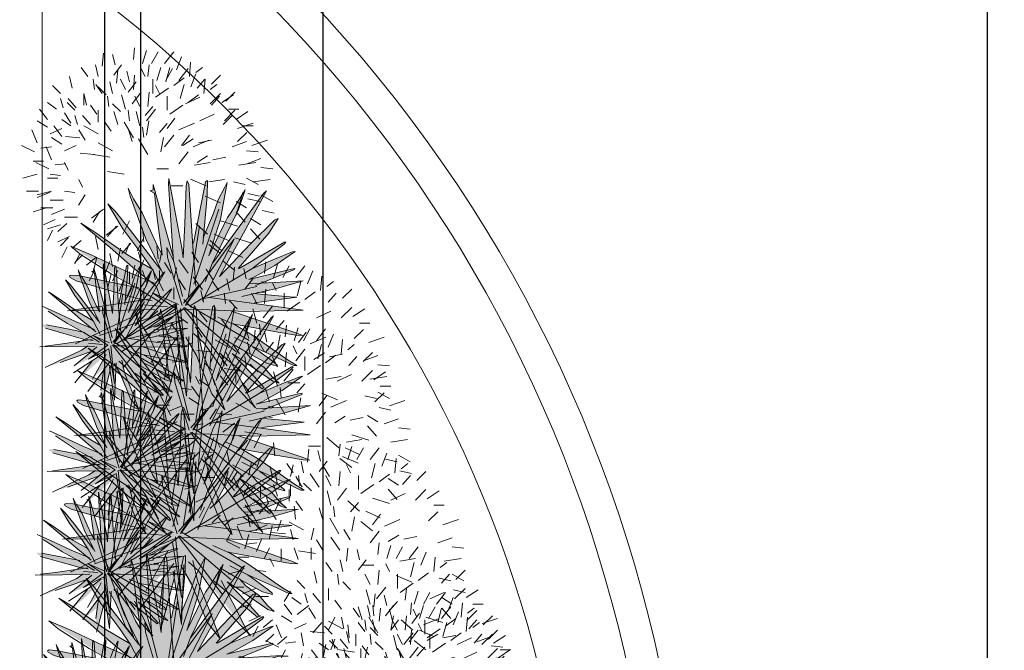
# Model space of a CAD drawing. Units: inches. Extents: x 1239 to 2276906, y 2273 to 321338.
# Tile 7 of 23: x 1541 to 1664, y 2428 to 2507. Entities that reach past the tile are written whole.
import ezdxf

# ---------------------------------------------------------------- set-up
doc = ezdxf.new("R2010")
doc.units = ezdxf.units.IN
doc.layers.add('A-ANNO-DIMS', color=2, linetype='Continuous', lineweight=18)
doc.layers.add('L-PLNT', color=94, linetype='Continuous', lineweight=13)
doc.styles.get("Standard").update_dxf_attribs({"font": 'arial.ttf'})
doc.dimstyles.new('ISO-25', dxfattribs={"dimtxt": 4.5, "dimasz": 4, "dimexe": 1.25, "dimexo": 0.625, "dimtad": 1, "dimdec": 1, "dimlunit": 3, "dimtxsty": 'Standard', "dimcen": 2.5, "dimadec": 0, "dimazin": 0, "dimtfac": 1, "dimtdec": 1, "dimtmove": 0, "dimatfit": 3, "dimfxl": 1, "dimarcsym": 0})

# ---------------------------------------------------------------- blocks, each defined once
blk = doc.blocks.new('A$C545C060E')
h = blk.add_hatch(color=256)
h.set_gradient(color1=(31, 127, 0), color2=(45, 179, 0), one_color=1, tint=0.35, name='INVSPHERICAL')
h.paths.add_polyline_path([(0.529, 2.393), (0.645, 2.304), (1.889, 1.967), (0.489, 1.77), (1.843, 1.787), (1.618, 1.643), (0.635, 1.178), (1.063, 1.326), (1.966, 1.643), (1.461, 1.231), (1.869, 1.417), (2.379, 1.664), (2.177, 1.5), (1.446, 1.03), (1.981, 1.358), (1.481, 0.744), (2.376, 1.553), (1.986, 0.848), (2.48, 1.336), (1.85, 0.496), (2.266, 0.842), (2.223, 0.533), (2.243, 0.142), (2.487, 1.093), (2.615, 0.257), (2.655, 1.214), (3.074, 0.284), (3.303, 0), (2.908, 1.003), (2.846, 1.271), (2.929, 1.199), (3.853, 0.038), (3.428, 0.832), (3.973, 0.376), (4.009, 0.393), (3.432, 1.008), (3.923, 0.676), (4.175, 0.507), (4.274, 0.474), (4.155, 0.583), (4.009, 0.757), (3.765, 0.932), (3.662, 1.051), (4.067, 0.828), (4.243, 0.779), (4.238, 0.801), (3.802, 1.133), (4.534, 0.795), (4.591, 0.795), (4.42, 0.899), (4.103, 1.12), (3.786, 1.34), (3.464, 1.533), (3.968, 1.441), (4.415, 1.362), (4.571, 1.335), (4.695, 1.33), (3.997, 1.572), (3.423, 1.771), (4.695, 1.782), (3.833, 1.912), (4.591, 2.011), (3.836, 2.079), (4.706, 2.305), (3.951, 2.263), (4.55, 2.506), (4.555, 2.528), (4.493, 2.517), (3.734, 2.332), (4.197, 2.577), (4.56, 2.833), (3.786, 2.523), (4.363, 2.959), (4.394, 2.997), (4.363, 2.997), (3.558, 2.528), (3.549, 2.536), (4.087, 3.155), (4.254, 3.422), (4.191, 3.389), (3.209, 2.381), (4.046, 3.912), (3.999, 3.874), (3.09, 2.626), (3.547, 3.58), (3.666, 3.934), (3.35, 3.438), (3.017, 2.752), (3.225, 3.411), (3.345, 4.064), (3.243, 3.868), (3.184, 3.754), (2.919, 3.073), (2.986, 3.83), (2.991, 4.097), (2.96, 4.075), (2.742, 2.981), (2.732, 2.92), (2.659, 4.026), (2.633, 4.092), (2.612, 4.005), (2.56, 2.719), (2.3, 4.135), (2.382, 2.743), (2.025, 4.026), (2.02, 3.934), (1.968, 3.917), (2.046, 3.874), (2.185, 2.776), (1.976, 3.197), (1.829, 3.524), (1.673, 3.773), (1.577, 3.963), (1.613, 3.821), (1.751, 3.44), (1.89, 3.059), (2.192, 2.446), (1.345, 3.551), (1.215, 3.683), (1.481, 3.234), (2.006, 2.515), (1.567, 2.769), (0.983, 3.176), (0.731, 3.334), (1.255, 2.901), (1.969, 2.294), (0.912, 2.769), (0.549, 2.927), (1.687, 2.199), (0.675, 2.399), (0.554, 2.409)])
h = blk.add_hatch(color=256)
h.set_gradient(color1=(31, 127, 0), color2=(55, 219, 0), one_color=1, tint=0.43, name='SPHERICAL')
h.paths.add_polyline_path([(3.023, 2.188), (3.114, 2.362), (3.471, 3.049), (3.33, 2.866), (2.618, 1.891), (2.679, 1.855), (2.94, 2.013)])
h = blk.add_hatch(color=256)
h.set_gradient(color1=(31, 127, 0), color2=(45, 179, 0), one_color=1, tint=0.35, name='INVSPHERICAL')
h.paths.add_polyline_path([(0.025, 1.517), (0.098, 1.461), (0.877, 1.25), (0, 1.126), (0.848, 1.137), (0.707, 1.047), (0.092, 0.756), (0.36, 0.848), (0.925, 1.047), (0.609, 0.789), (0.865, 0.905), (1.184, 1.06), (1.058, 0.958), (0.6, 0.663), (0.935, 0.868), (0.622, 0.484), (1.182, 0.99), (0.938, 0.549), (1.247, 0.855), (0.853, 0.328), (1.113, 0.545), (1.086, 0.352), (1.099, 0.106), (1.252, 0.703), (1.332, 0.179), (1.357, 0.779), (1.62, 0.195), (1.763, 0.018), (1.515, 0.646), (1.477, 0.814), (1.529, 0.769), (2.108, 0.042), (1.841, 0.539), (2.183, 0.253), (2.206, 0.264), (1.844, 0.649), (2.152, 0.441), (2.31, 0.335), (2.371, 0.315), (2.297, 0.383), (2.206, 0.492), (2.053, 0.602), (1.988, 0.676), (2.242, 0.537), (2.352, 0.506), (2.349, 0.52), (2.076, 0.728), (2.534, 0.516), (2.57, 0.516), (2.463, 0.581), (2.264, 0.719), (2.066, 0.857), (1.864, 0.978), (2.18, 0.921), (2.46, 0.871), (2.557, 0.854), (2.636, 0.851), (2.198, 1.003), (1.839, 1.127), (2.636, 1.134), (2.095, 1.216), (2.57, 1.277), (2.097, 1.32), (2.642, 1.462), (2.169, 1.435), (2.544, 1.588), (2.548, 1.602), (2.509, 1.595), (2.033, 1.479), (2.323, 1.632), (2.551, 1.793), (2.066, 1.598), (2.427, 1.871), (2.447, 1.895), (2.427, 1.895), (1.923, 1.602), (1.917, 1.606), (2.255, 1.994), (2.359, 2.161), (2.32, 2.141), (1.704, 1.509), (2.229, 2.469), (2.199, 2.445), (1.63, 1.663), (1.916, 2.26), (1.991, 2.482), (1.792, 2.172), (1.584, 1.741), (1.714, 2.155), (1.789, 2.564), (1.726, 2.441), (1.688, 2.369), (1.522, 1.943), (1.565, 2.417), (1.568, 2.584), (1.548, 2.571), (1.412, 1.885), (1.405, 1.847), (1.36, 2.54), (1.343, 2.581), (1.33, 2.526), (1.298, 1.721), (1.135, 2.608), (1.186, 1.736), (0.962, 2.54), (0.959, 2.482), (0.927, 2.472), (0.976, 2.445), (1.063, 1.757), (0.932, 2.02), (0.84, 2.226), (0.742, 2.381), (0.682, 2.501), (0.704, 2.411), (0.791, 2.173), (0.878, 1.934), (1.067, 1.55), (0.537, 2.242), (0.455, 2.325), (0.622, 2.044), (0.951, 1.593), (0.676, 1.752), (0.31, 2.007), (0.152, 2.107), (0.48, 1.835), (0.927, 1.455), (0.265, 1.752), (0.038, 1.851), (0.751, 1.395), (0.117, 1.52), (0.041, 1.527)])
h = blk.add_hatch(color=256)
h.set_gradient(color1=(31, 127, 0), color2=(55, 219, 0), one_color=1, tint=0.43, name='SPHERICAL')
h.paths.add_polyline_path([(1.334, 1.202), (1.372, 1.18), (1.536, 1.279), (1.588, 1.388), (1.645, 1.497), (1.868, 1.928), (1.78, 1.813)])
for p, q in [((2.295, 4.037, -52.769), (2.3, 4.135, -52.769)), ((2.3, 4.135, -52.769), (2.534, 2.893, -52.769)), ((2.612, 4.005, -52.769), (2.633, 4.092, -52.769)), ((2.633, 4.092, -52.769), (2.659, 4.026, -52.769)), ((2.945, 4.01, -52.769), (2.96, 4.075, -52.769)), ((2.96, 4.075, -52.769), (2.991, 4.097, -52.769)), ((2.991, 4.097, -52.769), (2.986, 3.83, -52.769)), ((3.345, 4.064, -52.769), (3.225, 3.411, -52.769)), ((3.303, 3.983, -52.769), (3.345, 4.064, -52.769)), ((1.577, 3.963, -52.769), (1.613, 3.821, -52.769)), ((1.673, 3.773, -52.769), (1.577, 3.963, -52.769)), ((1.968, 3.917, -52.769), (2.02, 3.934, -52.769)), ((2.046, 3.874, -52.769), (1.968, 3.917, -52.769)), ((2.02, 3.934, -52.769), (2.025, 4.026, -52.769)), ((2.025, 4.026, -52.769), (2.389, 2.719, -52.769)), ((2.103, 3.378, -52.769), (2.046, 3.874, -52.769)), ((2.389, 2.643, -52.769), (2.295, 4.037, -52.769)), ((2.591, 3.329, -52.769), (2.612, 4.005, -52.769)), ((2.659, 4.026, -52.769), (2.732, 2.92, -52.769)), ((2.742, 2.981, -52.769), (2.945, 4.01, -52.769)), ((3.184, 3.754, -52.769), (3.303, 3.983, -52.769)), ((3.428, 3.553, -52.769), (3.666, 3.934, -52.769)), ((3.508, 3.479, -52.769), (3.625, 3.884, -52.769)), ((3.666, 3.934, -52.769), (3.547, 3.58, -52.769)), ((3.558, 3.269, -52.769), (3.999, 3.874, -52.769)), ((4.046, 3.912, -52.769), (3.635, 3.155, -52.769)), ((3.999, 3.874, -52.769), (4.046, 3.912, -52.769)), ((1.613, 3.821, -52.769), (1.89, 3.059, -52.769)), ((1.829, 3.524, -52.769), (1.673, 3.773, -52.769)), ((2.986, 3.83, -52.769), (2.908, 2.964, -52.769)), ((3.095, 3.498, -52.769), (3.184, 3.754, -52.769)), ((1.215, 3.683, -52.769), (1.481, 3.234, -52.769)), ((1.345, 3.551, -52.769), (1.215, 3.683, -52.769)), ((1.602, 3.229, -52.769), (1.345, 3.551, -52.769)), ((1.976, 3.197, -52.769), (1.829, 3.524, -52.769)), ((3.198, 3.588, -52.769), (2.75, 2.248, -52.769)), ((3.547, 3.58, -52.769), (3.085, 2.626, -52.769)), ((3.35, 3.438, -52.769), (3.428, 3.553, -52.769)), ((2.186, 2.773, -52.769), (2.103, 3.378, -52.769)), ((2.919, 3.073, -52.769), (3.095, 3.498, -52.769)), ((3.225, 3.411, -52.769), (3.017, 2.752, -52.769)), ((3.298, 3.329, -52.769), (3.35, 3.438, -52.769)), ((3.771, 2.975, -52.769), (4.191, 3.389, -52.769)), ((4.254, 3.422, -52.769), (4.087, 3.155, -52.769)), ((4.191, 3.389, -52.769), (4.254, 3.422, -52.769)), ((0.731, 3.334, -52.769), (1.255, 2.901, -52.769)), ((0.983, 3.176, -52.769), (0.731, 3.334, -52.769)), ((1.567, 2.769, -52.769), (0.983, 3.176, -52.769)), ((1.481, 3.234, -52.769), (1.819, 2.785, -52.769)), ((2.157, 2.505, -52.769), (1.602, 3.229, -52.769)), ((2.102, 2.927, -52.769), (1.976, 3.197, -52.769)), ((2.56, 2.719, -52.769), (2.591, 3.329, -52.769)), ((2.849, 3.284, -52.769), (2.65, 1.996, -52.769)), ((3.017, 2.752, -52.769), (3.298, 3.329, -52.769)), ((3.09, 2.626, -52.769), (3.558, 3.269, -52.769)), ((1.89, 3.059, -52.769), (2.192, 2.446, -52.769)), ((3.471, 3.049, -52.769), (3.114, 2.362, -52.769)), ((3.635, 3.155, -52.769), (3.209, 2.381, -52.769)), ((3.33, 2.866, -52.769), (3.471, 3.049, -52.769)), ((4.087, 3.155, -52.769), (3.542, 2.528, -52.769)), ((4.327, 2.975, -52.769), (4.363, 2.997, -52.769)), ((4.394, 2.997, -52.769), (4.363, 2.959, -52.769)), ((4.363, 2.997, -52.769), (4.394, 2.997, -52.769)), ((0.549, 2.927, -52.769), (0.72, 2.785, -52.769)), ((0.912, 2.769, -52.769), (0.549, 2.927, -52.769)), ((1.255, 2.901, -52.769), (1.653, 2.552, -52.769)), ((2.192, 2.764, -52.769), (2.102, 2.927, -52.769)), ((2.269, 2.899, -52.769), (2.394, 2.654, -52.769)), ((2.279, 2.724, -52.769), (2.269, 2.899, -52.769)), ((2.534, 2.893, -52.769), (2.56, 2.719, -52.769)), ((2.6, 1.866, -52.769), (3.33, 2.866, -52.769)), ((2.732, 2.92, -52.769), (2.783, 2.212, -52.769)), ((3.209, 2.381, -52.769), (3.771, 2.975, -52.769)), ((3.558, 2.528, -52.769), (4.327, 2.975, -52.769)), ((4.363, 2.959, -52.769), (3.786, 2.523, -52.769)), ((4.191, 2.692, -52.769), (4.514, 2.822, -52.769)), ((4.56, 2.833, -52.769), (4.197, 2.577, -52.769)), ((4.514, 2.822, -52.769), (4.56, 2.833, -52.769)), ((0.72, 2.785, -52.769), (1.27, 2.43, -52.769)), ((1.522, 2.483, -52.769), (0.912, 2.769, -52.769)), ((2.006, 2.515, -52.769), (1.567, 2.769, -52.769)), ((1.819, 2.785, -52.769), (2.016, 2.494, -52.769)), ((2.539, 1.864, -52.769), (2.279, 2.724, -52.769)), ((2.394, 2.654, -52.769), (2.55, 2.027, -52.769)), ((3.797, 2.528, -52.769), (4.191, 2.692, -52.769)), ((0.682, 2.501), (0.704, 2.411)), ((0.742, 2.381), (0.682, 2.501)), ((0.927, 2.472), (0.959, 2.482)), ((0.976, 2.445), (0.927, 2.472)), ((0.959, 2.482), (0.962, 2.54)), ((0.962, 2.54), (1.19, 1.721)), ((1.132, 2.547), (1.135, 2.608)), ((1.19, 1.673), (1.132, 2.547)), ((1.135, 2.608), (1.281, 1.83)), ((1.317, 2.103), (1.33, 2.526)), ((1.33, 2.526), (1.343, 2.581)), ((1.343, 2.581), (1.36, 2.54)), ((1.36, 2.54), (1.405, 1.847)), ((1.412, 1.885), (1.539, 2.53)), ((2.046, 2.261, -52.769), (1.522, 2.483, -52.769)), ((1.539, 2.53), (1.548, 2.571)), ((1.548, 2.571), (1.568, 2.584)), ((1.568, 2.584), (1.565, 2.417)), ((1.653, 2.552, -52.769), (2.087, 2.198, -52.769)), ((1.688, 2.369), (1.763, 2.513)), ((1.789, 2.564), (1.714, 2.155)), ((1.763, 2.513), (1.789, 2.564)), ((1.841, 2.243), (1.991, 2.482)), ((1.991, 2.482), (1.916, 2.26)), ((2.229, 2.469), (1.971, 1.994)), ((2.016, 2.494, -52.769), (2.208, 2.129, -52.769)), ((2.199, 2.445), (2.229, 2.469)), ((3.786, 2.523, -52.769), (2.674, 1.853, -52.769)), ((3.085, 2.626, -52.769), (2.955, 2.288, -52.769)), ((3.734, 2.332, -52.769), (4.493, 2.517, -52.769)), ((4.197, 2.577, -52.769), (3.848, 2.381, -52.769)), ((4.55, 2.506, -52.769), (3.854, 2.223, -52.769)), ((4.493, 2.517, -52.769), (4.555, 2.528, -52.769)), ((4.555, 2.528, -52.769), (4.55, 2.506, -52.769)), ((0.455, 2.325), (0.622, 2.044)), ((0.537, 2.242), (0.455, 2.325)), ((0.554, 2.409, -52.769), (0.529, 2.393, -52.769)), ((0.529, 2.393, -52.769), (0.539, 2.367, -52.769)), ((0.539, 2.367, -52.769), (0.645, 2.304, -52.769)), ((0.675, 2.399, -52.769), (0.554, 2.409, -52.769)), ((0.645, 2.304, -52.769), (1.734, 1.992, -52.769)), ((1.32, 2.272, -52.769), (0.675, 2.399, -52.769)), ((0.704, 2.411), (0.878, 1.934)), ((0.84, 2.226), (0.742, 2.381)), ((1.011, 2.134), (0.976, 2.445)), ((1.27, 2.43, -52.769), (1.764, 2.156, -52.769)), ((1.565, 2.417), (1.516, 1.875)), ((1.633, 2.209), (1.688, 2.369)), ((1.891, 2.197), (1.965, 2.451)), ((1.923, 2.066), (2.199, 2.445)), ((3.114, 2.362, -52.769), (3.023, 2.188, -52.769)), ((3.848, 2.381, -52.769), (3.734, 2.332, -52.769)), ((4.706, 2.305, -52.769), (4.228, 2.169, -52.769)), ((4.301, 2.283, -52.769), (4.706, 2.305, -52.769)), ((0.698, 2.04), (0.537, 2.242)), ((0.932, 2.02), (0.84, 2.226)), ((1.063, 1.755), (1.011, 2.134)), ((1.769, 2.182, -52.769), (1.32, 2.272, -52.769)), ((1.697, 2.266), (1.416, 1.426)), ((1.522, 1.943), (1.633, 2.209)), ((1.714, 2.155), (1.584, 1.741)), ((1.916, 2.26), (1.627, 1.663)), ((1.76, 2.103), (1.792, 2.172)), ((1.764, 2.156, -52.769), (2.182, 1.902, -52.769)), ((1.792, 2.172), (1.841, 2.243)), ((2.056, 1.881), (2.32, 2.141)), ((2.359, 2.161), (2.255, 1.994)), ((2.32, 2.141), (2.359, 2.161)), ((2.565, 1.907, -52.769), (2.84, 2.229, -52.769)), ((2.84, 2.229, -52.769), (2.606, 1.885, -52.769)), ((3.878, 2.205, -52.769), (2.857, 1.97, -52.769)), ((3.023, 2.188, -52.769), (2.907, 1.944, -52.769)), ((4.228, 2.169, -52.769), (3.61, 2.027, -52.769)), ((3.734, 2.25, -52.769), (4.301, 2.283, -52.769)), ((3.949, 2.282, -52.769), (4.001, 2.285, -52.769)), ((4.001, 2.285, -52.769), (4.042, 2.282, -52.769)), ((0.152, 2.107), (0.48, 1.835)), ((0.31, 2.007), (0.152, 2.107)), ((0.676, 1.752), (0.31, 2.007)), ((0.622, 2.044), (0.834, 1.762)), ((1.045, 1.587), (0.698, 2.04)), ((1.011, 1.851), (0.932, 2.02)), ((1.981, 1.981, -52.769), (1.068, 1.844, -52.769)), ((1.298, 1.721), (1.317, 2.103)), ((1.479, 2.075), (1.354, 1.268)), ((1.584, 1.741), (1.76, 2.103)), ((1.63, 1.663), (1.923, 2.066)), ((1.971, 1.994), (1.704, 1.509)), ((1.734, 1.992, -52.769), (2.006, 1.949, -52.769)), ((2.255, 1.994), (1.913, 1.602)), ((2.009, 2.092, -52.769), (2.476, 1.885, -52.769)), ((2.425, 1.814, -52.769), (2.009, 2.092, -52.769)), ((3.516, 1.945, -52.769), (3.028, 2.005, -52.769)), ((4.701, 1.782, -52.769), (3.516, 1.945, -52.769)), ((3.807, 2.082, -52.769), (4.264, 2.038, -52.769)), ((4.591, 2.011, -52.769), (3.833, 1.912, -52.769)), ((3.886, 2.102, -52.769), (3.98, 2.099, -52.769)), ((3.98, 2.099, -52.769), (4.025, 2.091, -52.769)), ((4.264, 2.038, -52.769), (4.534, 2.016, -52.769)), ((4.534, 2.016, -52.769), (4.591, 2.011, -52.769)), ((0.265, 1.752), (0.038, 1.851)), ((0.145, 1.762), (0.49, 1.54)), ((0.48, 1.835), (0.729, 1.617)), ((0.64, 1.791, -52.769), (0.489, 1.77, -52.769)), ((0.489, 1.77, -52.769), (1.275, 1.775, -52.769)), ((1.068, 1.844, -52.769), (0.64, 1.791, -52.769)), ((0.834, 1.762), (0.957, 1.58)), ((0.878, 1.934), (1.067, 1.55)), ((1.067, 1.749), (1.011, 1.851)), ((1.115, 1.834), (1.194, 1.68)), ((1.122, 1.724), (1.115, 1.834)), ((1.275, 1.775, -52.769), (2.051, 1.791, -52.769)), ((1.281, 1.83), (1.298, 1.721)), ((1.323, 1.186), (1.78, 1.813)), ((1.405, 1.847), (1.438, 1.404)), ((1.868, 1.928), (1.645, 1.497)), ((1.865, 1.801, -52.769), (1.678, 1.675, -52.769)), ((1.704, 1.509), (2.056, 1.881)), ((1.78, 1.813), (1.868, 1.928)), ((1.869, 1.417, -52.769), (2.425, 1.814, -52.769)), ((1.87, 1.874, -52.769), (2.276, 1.84, -52.769)), ((1.923, 1.602), (2.404, 1.881)), ((1.966, 1.643, -52.769), (2.107, 1.77, -52.769)), ((2.427, 1.871), (2.066, 1.598)), ((2.32, 1.704), (2.522, 1.786)), ((2.551, 1.793), (2.323, 1.632)), ((2.404, 1.881), (2.427, 1.895)), ((2.447, 1.895), (2.427, 1.871)), ((2.427, 1.895), (2.447, 1.895)), ((2.513, 1.809, -52.769), (2.617, 0.725, -52.769)), ((2.522, 1.786), (2.551, 1.793)), ((2.913, 1.793, -52.769), (2.555, 1.798, -52.769)), ((3.347, 0.787, -52.769), (2.559, 1.822, -52.769)), ((3.504, 1.039, -52.769), (2.584, 1.831, -52.769)), ((3.737, 1.239, -52.769), (2.617, 1.892, -52.769)), ((3.672, 1.76, -52.769), (2.913, 1.793, -52.769)), ((3.422, 1.766, -52.769), (4.571, 1.379, -52.769)), ((4.695, 1.782, -52.769), (3.672, 1.76, -52.769)), ((0.647, 1.573), (0.265, 1.752)), ((0.951, 1.593), (0.676, 1.752)), ((0.729, 1.617), (1.001, 1.395)), ((1.285, 1.185), (1.122, 1.724)), ((1.194, 1.68), (1.291, 1.288)), ((1.618, 1.643, -52.769), (1.345, 1.521, -52.769)), ((2.066, 1.598), (1.369, 1.178)), ((1.966, 1.643, -52.769), (1.461, 1.231, -52.769)), ((1.627, 1.663), (1.545, 1.451)), ((1.608, 1.516, -52.769), (1.966, 1.643, -52.769)), ((1.678, 1.675, -52.769), (1.618, 1.643, -52.769)), ((2.456, 1.716, -52.769), (1.869, 1.417, -52.769)), ((2.033, 1.479), (2.509, 1.595)), ((2.072, 1.602), (2.32, 1.704)), ((2.323, 1.632), (2.105, 1.509)), ((2.544, 1.588), (2.108, 1.41)), ((2.177, 1.5, -52.769), (2.379, 1.664, -52.769)), ((2.617, 0.725, -52.769), (2.456, 1.716, -52.769)), ((2.509, 1.595), (2.548, 1.602)), ((2.548, 1.602), (2.544, 1.588)), ((3.443, 1.537, -52.769), (3.178, 1.657, -52.769)), ((0.098, 1.461), (0.78, 1.265)), ((0.521, 1.441), (0.117, 1.52)), ((0.49, 1.54), (0.799, 1.368)), ((0.802, 1.385), (0.521, 1.441)), ((0.976, 1.434), (0.647, 1.573)), ((0.957, 1.58), (1.077, 1.352)), ((1.345, 1.521, -52.769), (1.048, 1.379, -52.769)), ((1.063, 1.326, -52.769), (1.608, 1.516, -52.769)), ((1.301, 1.212), (1.473, 1.414)), ((1.473, 1.414), (1.327, 1.199)), ((1.446, 1.03, -52.769), (2.177, 1.5, -52.769)), ((1.645, 1.497), (1.588, 1.388)), ((1.986, 0.848, -52.769), (2.376, 1.553, -52.769)), ((2.105, 1.509), (2.033, 1.479)), ((2.033, 1.427), (2.388, 1.448)), ((2.168, 1.447), (2.2, 1.449)), ((2.2, 1.449), (2.226, 1.447)), ((2.642, 1.462), (2.343, 1.376)), ((2.388, 1.448), (2.642, 1.462)), ((3.677, 1.493, -52.769), (3.443, 1.537, -52.769)), ((3.448, 1.542, -52.769), (3.786, 1.34, -52.769)), ((4.259, 1.39, -52.769), (3.677, 1.493, -52.769)), ((0.935, 1.259), (0.363, 1.173)), ((1.048, 1.379, -52.769), (0.635, 1.178, -52.769)), ((0.78, 1.265), (0.951, 1.239)), ((0.799, 1.368), (1.061, 1.209)), ((0.952, 1.328), (1.245, 1.199)), ((1.213, 1.154), (0.952, 1.328)), ((1.981, 1.358, -52.769), (1.481, 0.744, -52.769)), ((2.123, 1.399), (1.484, 1.252)), ((1.588, 1.388), (1.515, 1.235)), ((1.897, 1.236), (1.591, 1.274)), ((2.639, 1.134), (1.897, 1.236)), ((2.343, 1.376), (1.955, 1.288)), ((2.079, 1.322), (2.365, 1.294)), ((2.57, 1.277), (2.095, 1.216)), ((2.128, 1.335), (2.187, 1.333)), ((2.187, 1.333), (2.215, 1.328)), ((2.313, 1.109, -52.769), (2.48, 1.336, -52.769)), ((2.365, 1.294), (2.534, 1.281)), ((2.534, 1.281), (2.57, 1.277)), ((2.799, 0.97, -52.769), (2.606, 1.297, -52.769)), ((2.658, 1.308, -52.769), (2.617, 0.245, -52.769)), ((2.929, 1.199, -52.769), (2.742, 1.362, -52.769)), ((2.819, 1.39, -52.769), (2.908, 1.003, -52.769)), ((3.62, 1.074, -52.769), (3.313, 1.248, -52.769)), ((3.802, 1.133, -52.769), (3.479, 1.292, -52.769)), ((3.786, 1.34, -52.769), (4.42, 0.899, -52.769)), ((4.571, 1.335, -52.769), (4.259, 1.39, -52.769)), ((4.571, 1.379, -52.769), (4.695, 1.33, -52.769)), ((4.695, 1.33, -52.769), (4.571, 1.335, -52.769)), ((0, 1.126), (0.493, 1.13)), ((0.363, 1.173), (0.095, 1.14)), ((0.493, 1.13), (0.979, 1.14)), ((0.745, 1.067), (0.707, 1.047)), ((0.862, 1.146), (0.745, 1.067)), ((0.865, 0.905), (1.213, 1.154)), ((1.232, 1.093), (0.865, 0.905)), ((0.866, 1.192), (1.12, 1.17)), ((0.925, 1.047), (1.014, 1.126)), ((1.058, 0.958), (1.184, 1.06)), ((1.333, 0.472), (1.232, 1.093)), ((1.268, 1.151), (1.333, 0.472)), ((1.519, 1.141), (1.294, 1.144)), ((1.791, 0.511), (1.297, 1.159)), ((1.889, 0.669), (1.312, 1.165)), ((2.035, 0.794), (1.333, 1.203)), ((1.994, 1.12), (1.519, 1.141)), ((1.838, 1.124), (2.557, 0.881)), ((1.85, 0.496, -52.769), (2.313, 1.109, -52.769)), ((2.636, 1.134), (1.994, 1.12)), ((2.308, 1.151, -52.769), (2.223, 0.533, -52.769)), ((2.243, 0.142, -52.769), (2.485, 1.067, -52.769)), ((2.617, 0.245, -52.769), (2.471, 1.199, -52.769)), ((2.485, 1.067, -52.769), (2.5, 1.22, -52.769)), ((3.427, 0.496, -52.769), (2.929, 1.199, -52.769)), ((4.067, 0.828, -52.769), (3.62, 1.074, -52.769)), ((3.656, 1.057, -52.769), (3.765, 0.932, -52.769)), ((4.243, 0.932, -52.769), (3.802, 1.133, -52.769)), ((3.802, 1.128, -52.769), (4.176, 0.856, -52.769)), ((0.351, 0.881), (0.092, 0.756)), ((0.537, 0.971), (0.351, 0.881)), ((0.36, 0.848), (0.701, 0.967)), ((0.707, 1.047), (0.537, 0.971)), ((0.6, 0.663), (1.058, 0.958)), ((0.925, 1.047), (0.609, 0.789)), ((0.701, 0.967), (0.925, 1.047)), ((0.938, 0.549), (1.182, 0.99)), ((1.46, 0.888), (1.515, 0.646)), ((1.851, 0.98), (1.685, 1.056)), ((1.997, 0.953), (1.851, 0.98)), ((1.854, 0.984), (2.066, 0.857)), ((2.362, 0.888), (1.997, 0.953)), ((2.557, 0.854), (2.362, 0.888)), ((2.557, 0.881), (2.636, 0.851)), ((3.074, 0.284, -52.769), (2.799, 0.97, -52.769)), ((2.908, 1.003, -52.769), (3.111, 0.512, -52.769)), ((3.973, 0.376, -52.769), (3.204, 1.019, -52.769)), ((3.324, 1.03, -52.769), (3.599, 0.507, -52.769)), ((3.687, 0.839, -52.769), (3.432, 1.008, -52.769)), ((3.432, 1.008, -52.769), (3.786, 0.643, -52.769)), ((3.765, 0.932, -52.769), (4.009, 0.757, -52.769)), ((4.534, 0.795, -52.769), (4.243, 0.932, -52.769)), ((4.42, 0.899, -52.769), (4.591, 0.795, -52.769)), ((0.935, 0.868), (0.622, 0.484)), ((0.853, 0.328), (1.143, 0.713)), ((1.14, 0.739), (1.086, 0.352)), ((1.143, 0.713), (1.247, 0.855)), ((1.333, 0.171), (1.242, 0.769)), ((1.251, 0.686), (1.26, 0.782)), ((1.447, 0.625), (1.327, 0.83)), ((1.359, 0.837), (1.333, 0.171)), ((1.529, 0.769), (1.411, 0.871)), ((1.841, 0.328), (1.529, 0.769)), ((1.962, 0.69), (1.77, 0.799)), ((2.076, 0.728), (1.874, 0.827)), ((2.066, 0.857), (2.463, 0.581)), ((2.352, 0.602), (2.076, 0.728)), ((2.076, 0.724), (2.31, 0.554)), ((2.636, 0.851), (2.557, 0.854)), ((4.16, 0.512, -52.769), (3.687, 0.839, -52.769)), ((4.009, 0.757, -52.769), (4.155, 0.583, -52.769)), ((4.243, 0.779, -52.769), (4.067, 0.828, -52.769)), ((4.176, 0.856, -52.769), (4.238, 0.801, -52.769)), ((4.238, 0.801, -52.769), (4.243, 0.779, -52.769)), ((4.591, 0.795, -52.769), (4.534, 0.795, -52.769)), ((1.099, 0.106), (1.251, 0.686)), ((1.62, 0.195), (1.447, 0.625)), ((1.515, 0.646), (1.643, 0.339)), ((2.183, 0.253), (1.701, 0.656)), ((1.776, 0.663), (1.948, 0.335)), ((2.004, 0.543), (1.844, 0.649)), ((1.844, 0.649), (2.066, 0.421)), ((2.242, 0.537), (1.962, 0.69)), ((1.984, 0.68), (2.053, 0.602)), ((2.3, 0.339), (2.004, 0.543)), ((2.053, 0.602), (2.206, 0.492)), ((2.352, 0.506), (2.242, 0.537)), ((2.31, 0.554), (2.349, 0.52)), ((2.534, 0.516), (2.352, 0.602)), ((2.463, 0.581), (2.57, 0.516)), ((3.786, 0.643, -52.769), (4.009, 0.393, -52.769)), ((4.155, 0.583, -52.769), (4.274, 0.474, -52.769)), ((2.066, 0.421), (2.206, 0.264)), ((2.206, 0.492), (2.297, 0.383)), ((2.297, 0.383), (2.371, 0.315)), ((2.349, 0.52), (2.352, 0.506)), ((2.57, 0.516), (2.534, 0.516)), ((3.111, 0.512, -52.769), (3.303, 0, -52.769)), ((3.853, 0.038, -52.769), (3.427, 0.496, -52.769)), ((3.599, 0.507, -52.769), (3.786, 0.131, -52.769)), ((4.009, 0.393, -52.769), (3.973, 0.376, -52.769)), ((4.274, 0.474, -52.769), (4.16, 0.512, -52.769)), ((1.763, 0.018), (1.62, 0.195)), ((1.643, 0.339), (1.763, 0.018)), ((2.108, 0.042), (1.841, 0.328)), ((1.948, 0.335), (2.066, 0.1)), ((2.206, 0.264), (2.183, 0.253)), ((2.371, 0.315), (2.3, 0.339)), ((3.303, 0, -52.769), (3.074, 0.284, -52.769)), ((2.066, 0.1), (2.108, 0.042)), ((3.786, 0.131, -52.769), (3.853, 0.038, -52.769))]:
    blk.add_line(p, q)
blk = doc.blocks.new('t1')
at = {"xscale": 1200, "yscale": 1200, "zscale": 1200}
blk.add_blockref('A$C545C060E', (1649217, 160231), dxfattribs=at)
blk = doc.blocks.new('A$C20C17E7E')
for p, q in [((1.899, 5.117), (1.929, 5.423)), ((2.205, 5.147), (2.144, 5.393)), ((2.635, 5.271), (2.665, 5.546)), ((2.849, 5.179), (2.941, 5.485)), ((3.063, 5.179), (3.217, 5.455)), ((3.37, 5.179), (3.584, 5.455)), ((3.646, 5.025), (3.768, 5.332)), ((1.807, 4.871), (1.746, 5.147)), ((2.174, 4.903), (2.359, 5.147)), ((3.952, 4.871), (3.983, 5.21)), ((1.195, 4.597), (1.134, 4.871)), ((1.562, 4.871), (1.409, 5.086)), ((2.635, 4.565), (2.665, 4.903)), ((2.91, 4.871), (2.819, 5.056)), ((3.401, 4.749), (3.492, 5.086)), ((4.105, 4.964), (4.259, 5.086)), ((4.472, 4.688), (4.687, 4.903)), ((0.919, 4.474), (0.735, 4.658)), ((1.716, 4.565), (1.685, 4.81)), ((2.45, 4.565), (2.328, 4.81)), ((3.095, 4.474), (3.095, 4.81)), ((3.584, 4.658), (3.829, 4.841)), ((4.135, 4.597), (4.32, 4.81)), ((1.47, 4.198), (1.47, 4.474)), ((1.991, 4.443), (1.807, 4.627)), ((2.45, 4.106), (2.359, 4.443)), ((2.604, 4.228), (2.819, 4.504)), ((3.156, 4.382), (3.462, 4.597)), ((4.442, 4.228), (4.687, 4.474)), ((4.717, 4.259), (4.993, 4.443)), ((0.827, 4.106), (0.613, 4.259)), ((0.98, 4.137), (0.919, 4.352)), ((1.286, 4.137), (1.102, 4.352)), ((1.777, 3.983), (1.623, 4.198)), ((3.86, 4.228), (4.196, 4.382)), ((0.613, 3.861), (0.428, 4.106)), ((1.164, 3.77), (1.01, 4.014)), ((2.267, 3.739), (2.174, 4.045)), ((2.543, 3.831), (2.513, 4.076)), ((2.91, 3.953), (3.095, 4.167)), ((4.748, 3.739), (4.963, 3.953)), ((4.871, 4.106), (5.117, 4.106)), ((0.613, 3.677), (0.367, 3.831)), ((2.635, 3.431), (2.42, 3.8)), ((2.941, 3.494), (3.002, 3.831)), ((3.431, 3.646), (3.614, 3.892)), ((3.707, 3.616), (4.074, 3.77)), ((5.086, 3.646), (5.453, 3.77)), ((0.367, 3.31), (0.244, 3.616)), ((0.949, 3.646), (0.674, 3.524)), ((1.807, 3.524), (1.47, 3.707)), ((3.37, 3.218), (3.584, 3.494)), ((0.306, 3.095), (0, 3.249)), ((1.378, 3.431), (1.041, 3.463)), ((3.799, 3.249), (4.044, 3.401)), ((4.166, 3.31), (4.472, 3.37)), ((4.963, 3.218), (5.3, 3.34)), ((0.704, 3.218), (0.459, 3.188)), ((2.083, 2.973), (1.685, 3.034)), ((5.3, 3.125), (5.575, 3.095)), ((0.52, 2.88), (0.276, 2.88)), ((1.102, 2.666), (1.01, 2.849)), ((4.074, 2.788), (4.442, 2.849)), ((5.117, 2.788), (5.514, 2.849)), ((0.367, 2.574), (0.03, 2.482)), ((0.919, 2.543), (0.674, 2.574)), ((3.186, 2.697), (3.462, 2.697)), ((3.983, 2.452), (4.35, 2.298)), ((4.993, 2.391), (5.269, 2.33)), ((5.3, 2.482), (5.575, 2.33)), ((0.398, 2.176), (0.122, 2.176)), ((0.674, 2.145), (0.367, 2.022)), ((5.331, 2.115), (5.607, 2.054)), ((0.98, 1.961), (0.674, 1.961)), ((1.501, 2.084), (1.347, 1.839)), ((5.056, 1.931), (5.3, 1.778)), ((0.582, 1.778), (0.276, 1.685)), ((1.929, 1.748), (1.653, 1.533)), ((5.056, 1.685), (5.269, 1.44)), ((0.796, 1.502), (0.52, 1.379)), ((1.071, 1.409), (0.858, 1.226)), ((2.543, 1.472), (2.389, 1.164)), ((4.105, 1.409), (4.381, 1.164)), ((4.687, 1.472), (5.086, 1.348)), ((0.735, 1.257), (0.613, 1.012)), ((2.237, 1.348), (2.022, 1.103)), ((2.849, 1.287), (2.88, 0.981)), ((4.535, 1.164), (4.871, 1.012)), ((1.102, 1.073), (0.919, 0.888)), ((1.409, 1.012), (1.195, 0.827)), ((1.746, 1.103), (1.807, 0.797)), ((2.543, 0.951), (2.45, 0.705)), ((1.378, 0.705), (1.256, 0.46)), ((2.328, 0.827), (2.267, 0.521)), ((2.757, 0.736), (2.819, 0.491)), ((3.308, 0.766), (3.247, 0.491)), ((4.013, 0.736), (4.166, 0.491)), ((4.411, 0.92), (4.687, 0.705)), ((1.777, 0.614), (1.685, 0.276)), ((2.083, 0.521), (1.961, 0.215)), ((3.37, 0.491), (3.523, 0.245)), ((3.707, 0.552), (3.922, 0.245)), ((2.267, 0.306), (2.144, 0.062)), ((2.543, 0.276), (2.543, 0)), ((2.849, 0.306), (2.941, 0.03)), ((3.247, 0.306), (3.247, 0.03))]:
    blk.add_line(p, q)
blk = doc.blocks.new('*D58')
at = {"layer": 'A-ANNO-DIMS', "color": 0, "lineweight": -2, "transparency": 16777216}
for p, q in [((1701.17, 2606.31), (1674.02, 2606.31)), ((1675.27, 2602.31), (1675.27, 2433.5)), ((1701.17, 2429.5), (1674.02, 2429.5))]:
    blk.add_line(p, q, dxfattribs=at)
at = {"layer": 'A-ANNO-DIMS', "color": 0, "transparency": 16777216}
for points in [[(1674.61, 2602.31), (1675.94, 2602.31), (1675.27, 2606.31)], [(1674.61, 2433.5), (1675.94, 2433.5), (1675.27, 2429.5)]]:
    blk.add_solid(points, dxfattribs=at)
at = {"layer": 'Defpoints', "color": 0, "transparency": 16777216}
for p in [(1701.8, 2606.31), (1675.27, 2429.5), (1701.8, 2429.5)]:
    blk.add_point(p, dxfattribs=at)
at = {"layer": 'A-ANNO-DIMS', "color": 0, "transparency": 16777216, "insert": (1672.32, 2517.91), "char_height": 4.5, "attachment_point": 5, "rotation": 90}
blk.add_mtext('CAR 14\'-9" TYP.', dxfattribs=at)
blk = doc.blocks.new('*D89')
at = {"layer": 'A-ANNO-DIMS', "color": 0, "lineweight": -2, "transparency": 16777216}
for p, q in [((1359.38, 3215.77), (1359.38, 2275.7)), ((1551.38, 3215.77), (1551.38, 2275.7)), ((1363.38, 2276.95), (1547.38, 2276.95))]:
    blk.add_line(p, q, dxfattribs=at)
at = {"layer": 'A-ANNO-DIMS', "color": 0, "transparency": 16777216}
for points in [[(1363.38, 2277.61), (1363.38, 2276.28), (1359.38, 2276.95)], [(1547.38, 2277.61), (1547.38, 2276.28), (1551.38, 2276.95)]]:
    blk.add_solid(points, dxfattribs=at)
at = {"layer": 'Defpoints', "color": 0, "transparency": 16777216}
for p in [(1359.38, 3216.4), (1551.38, 3216.4), (1551.38, 2276.95)]:
    blk.add_point(p, dxfattribs=at)
at = {"layer": 'A-ANNO-DIMS', "color": 0, "transparency": 16777216, "insert": (1455.38, 2279.87), "char_height": 4.5, "attachment_point": 5}
blk.add_mtext('16\'-0"', dxfattribs=at)
blk = doc.blocks.new('*D96')
at = {"layer": 'A-ANNO-DIMS', "color": 0, "lineweight": -2, "transparency": 16777216}
for p, q in [((1555.88, 2629.77), (1555.88, 2275.7)), ((1661.88, 2629.77), (1661.88, 2275.7)), ((1559.88, 2276.95), (1657.88, 2276.95))]:
    blk.add_line(p, q, dxfattribs=at)
at = {"layer": 'A-ANNO-DIMS', "color": 0, "transparency": 16777216}
for points in [[(1559.88, 2277.61), (1559.88, 2276.28), (1555.88, 2276.95)], [(1657.88, 2277.61), (1657.88, 2276.28), (1661.88, 2276.95)]]:
    blk.add_solid(points, dxfattribs=at)
at = {"layer": 'Defpoints', "color": 0, "transparency": 16777216}
for p in [(1555.88, 2630.4), (1661.88, 2630.4), (1661.88, 2276.95)]:
    blk.add_point(p, dxfattribs=at)
at = {"layer": 'A-ANNO-DIMS', "color": 0, "transparency": 16777216, "insert": (1608.88, 2279.87), "char_height": 4.5, "attachment_point": 5}
blk.add_mtext('8\'-10"', dxfattribs=at)
blk = doc.blocks.new('*D112')
at = {"layer": 'A-ANNO-DIMS', "color": 0, "lineweight": -2, "transparency": 16777216}
for p, q in [((1555.88, 3371.77), (1555.88, 2275.7)), ((1661.88, 3371.77), (1661.88, 2275.7)), ((1559.88, 2276.95), (1657.88, 2276.95))]:
    blk.add_line(p, q, dxfattribs=at)
at = {"layer": 'A-ANNO-DIMS', "color": 0, "transparency": 16777216}
for points in [[(1559.88, 2277.61), (1559.88, 2276.28), (1555.88, 2276.95)], [(1657.88, 2277.61), (1657.88, 2276.28), (1661.88, 2276.95)]]:
    blk.add_solid(points, dxfattribs=at)
at = {"layer": 'Defpoints', "color": 0, "transparency": 16777216}
for p in [(1555.88, 3372.4), (1661.88, 3372.4), (1661.88, 2276.95)]:
    blk.add_point(p, dxfattribs=at)
at = {"layer": 'A-ANNO-DIMS', "color": 0, "transparency": 16777216, "insert": (1608.88, 2279.87), "char_height": 4.5, "attachment_point": 5}
blk.add_mtext('8\'-10"', dxfattribs=at)
blk = doc.blocks.new('*D114')
at = {"layer": 'A-ANNO-DIMS', "color": 0, "lineweight": -2, "transparency": 16777216}
for p, q in [((1555.88, 2850.27), (1555.88, 2275.7)), ((1578.7, 2850.27), (1578.7, 2275.7)), ((1559.88, 2276.95), (1574.7, 2276.95))]:
    blk.add_line(p, q, dxfattribs=at)
at = {"layer": 'A-ANNO-DIMS', "color": 0, "transparency": 16777216}
for points in [[(1559.88, 2277.61), (1559.88, 2276.28), (1555.88, 2276.95)], [(1574.7, 2277.61), (1574.7, 2276.28), (1578.7, 2276.95)]]:
    blk.add_solid(points, dxfattribs=at)
at = {"layer": 'Defpoints', "color": 0, "transparency": 16777216}
for p in [(1555.88, 2850.9), (1578.7, 2850.9), (1578.7, 2276.95)]:
    blk.add_point(p, dxfattribs=at)
at = {"layer": 'A-ANNO-DIMS', "color": 0, "transparency": 16777216, "insert": (1567.29, 2279.83), "char_height": 4.5, "attachment_point": 5}
blk.add_mtext('1\'-11"', dxfattribs=at)

msp = doc.modelspace()

# ---------------------------------------------------------------- linework, layer by layer
at = {"layer": 'L-PLNT'}
msp.add_line((1543.55, 2607.52), (1543.55, 2349.9), dxfattribs=at)
for centre, radius, start, end in [((1451.32, 2390.4), 173.37, 346.4906, 57.0041), ((1451.32, 2390.4), 169.37, 346.1653, 57.0041), ((1459.68, 2390.4), 150.37, 344.3754, 56.1007)]:
    msp.add_arc(centre, radius, start, end, dxfattribs=at)

# ---------------------------------------------------------------- block references
for name, p, xscale, yscale, zscale in [('A$C20C17E7E', (1540.96, 2474.27), 5.31977792485371, 5.31977792485371, 5.31977792485371), ('A$C20C17E7E', (1542.76, 2472.15), 5.31977792485371, 5.31977792485371, 5.31977792485371), ('t1', (-8085.11, 1522.99, 369.69), 0.0058381603033249, 0.0058381603033249, 0.0058381603033249), ('A$C20C17E7E', (1557.38, 2447.47), 5.31977792485371, 5.31977792485371, 5.31977792485371), ('t1', (-8084.2, 1507.37, 369.69), 0.0058381603033249, 0.0058381603033249, 0.0058381603033249), ('A$C20C17E7E', (1559.97, 2439.55), 5.31977792485371, 5.31977792485371, 5.31977792485371), ('t1', (-8085.73, 1494.4, 369.69), 0.0058381603033249, 0.0058381603033249, 0.0058381603033249), ('A$C20C17E7E', (1566.68, 2424.65), 5.31977792485371, 5.31977792485371, 5.31977792485371), ('A$C20C17E7E', (1571.57, 2412.27), 5.31977792485371, 5.31977792485371, 5.31977792485371), ('t1', (-8087.86, 1476.06, 369.69), 0.0058381603033249, 0.0058381603033249, 0.0058381603033249), ('A$C20C17E7E', (1574.99, 2406.56), 5.31977792485371, 5.31977792485371, 5.31977792485371), ('A$C20C17E7E', (1575.64, 2404.77), 5.31977792485371, 5.31977792485371, 5.31977792485371)]:
    msp.add_blockref(name, p, dxfattribs=dict(at, xscale=xscale, yscale=yscale, zscale=zscale))

# ---------------------------------------------------------------- dimensions: what is measured, and where the dimension line sits
at = {"layer": 'A-ANNO-DIMS'}
for base, p1, p2, picture, middle in [((1661.88, 2276.95), (1555.88, 3372.4), (1661.88, 3372.4), '*D112', (1608.88, 2279.87)), ((1551.38, 2276.95), (1359.38, 3216.4), (1551.38, 3216.4), '*D89', (1455.38, 2279.87)), ((1578.7, 2276.95), (1555.88, 2850.9), (1578.7, 2850.9), '*D114', (1567.29, 2279.83)), ((1661.88, 2276.95), (1555.88, 2630.4), (1661.88, 2630.4), '*D96', (1608.88, 2279.87))]:
    dim = msp.add_linear_dim(base=base, p1=p1, p2=p2, dimstyle='ISO-25', override={"dimdec": 1, "dimlfac": 1, "dimrnd": 0, "dimzin": 1, "dimdsep": 46, "dimlunit": 4, "dimfrac": 2}, dxfattribs=at)
    dim.commit()
    dim.dimension.update_dxf_attribs({"geometry": picture, "text_midpoint": middle})
dim = msp.add_linear_dim(base=(1675.27, 2429.5), p1=(1701.8, 2606.31), p2=(1701.8, 2429.5), angle=270, text='CAR <> TYP.', dimstyle='ISO-25', override={"dimdec": 1, "dimlfac": 1, "dimrnd": 0, "dimzin": 1, "dimdsep": 46, "dimlunit": 4, "dimfrac": 2}, dxfattribs=at)
dim.commit()
dim.dimension.update_dxf_attribs({"geometry": '*D58', "text_midpoint": (1672.32, 2517.91)})

doc.saveas('drawing.dxf')
